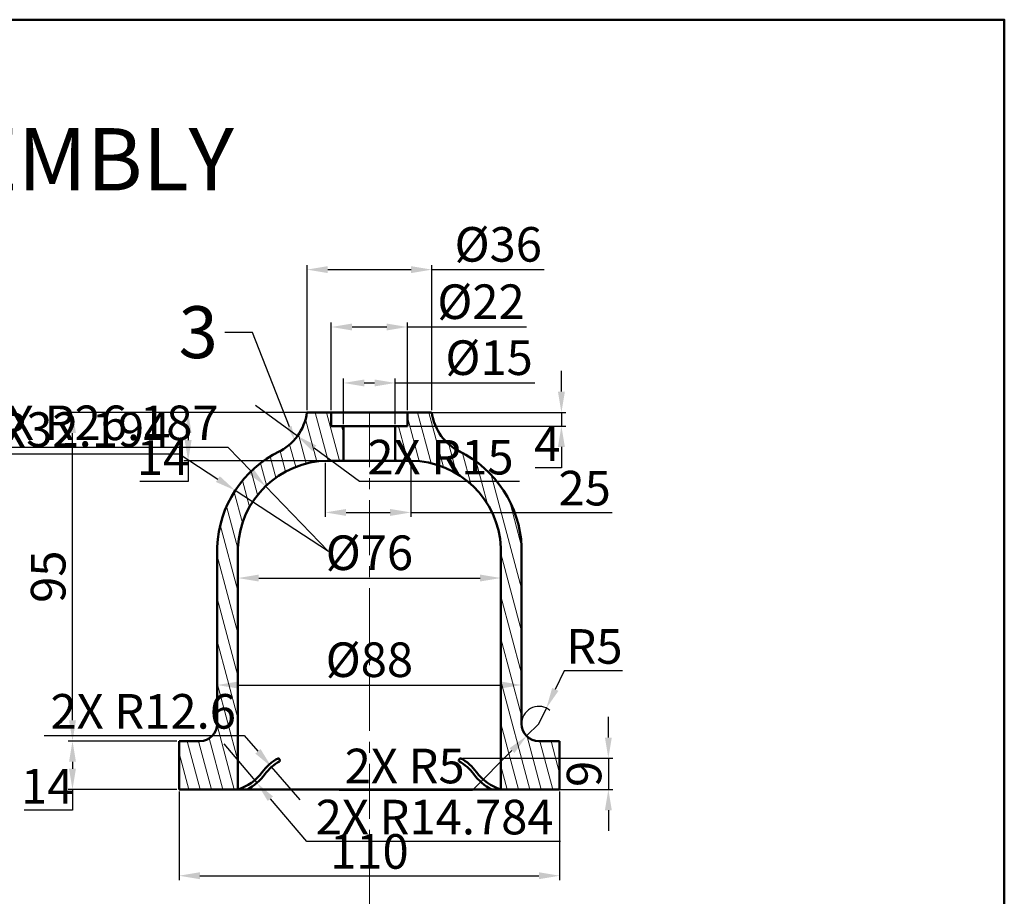
# Model space of a CAD drawing. Units: millimetres. Extents: x 147 to 984, y -369 to 435.
# Tile 10 of 10: x 699 to 984, y 182 to 435. Entities that reach past the tile are written whole.
import ezdxf
from ezdxf import colors
from ezdxf.entities.mleader import LeaderData, LeaderLine
from ezdxf.math import Vec2, Vec3

# ---------------------------------------------------------------- set-up
doc = ezdxf.new("R2010")
doc.units = ezdxf.units.MM
doc.header["$LTSCALE"] = 0.5
doc.linetypes.add('CENTER', pattern=[50.8, 31.75, -6.35, 6.35, -6.35])
for name, color, linetype, lineweight in [('M-CNTR', 1, 'CENTER', 18), ('M-DIMS', 2, 'Continuous', 25), ('M-HATC', 8, 'Continuous', 18), ('M-OUTL', 7, 'Continuous', 50), ('M-TEXT', 7, 'Continuous', 25)]:
    doc.layers.add(name, color=color, linetype=linetype, lineweight=lineweight)
doc.styles.get("Standard").update_dxf_attribs({"font": 'arial.ttf'})
doc.dimstyles.new('ISO-25', dxfattribs={"dimtxt": 10, "dimasz": 6, "dimexe": 1.25, "dimexo": 0.625, "dimtad": 1, "dimtoh": 1, "dimdec": 0, "dimtxsty": 'Standard', "dimcen": 2.5, "dimadec": 0, "dimazin": 0, "dimtfac": 1, "dimtdec": 0, "dimtmove": 0, "dimatfit": 3, "dimfxl": 1, "dimarcsym": 0})

# ---------------------------------------------------------------- blocks, each defined once
blk = doc.blocks.new('*D45')
at = {"layer": 'Defpoints', "color": 0, "transparency": 16777216}
for p in [(745.56, 212.8), (855.56, 212.8), (855.56, 187.86)]:
    blk.add_point(p, dxfattribs=at)
at = {"layer": 'M-DIMS', "color": 0, "lineweight": -2, "transparency": 16777216}
for p, q in [((745.56, 212.17), (745.56, 186.61)), ((855.56, 212.17), (855.56, 186.61)), ((751.56, 187.86), (849.56, 187.86))]:
    blk.add_line(p, q, dxfattribs=at)
at = {"layer": 'M-DIMS', "color": 0, "transparency": 16777216}
for points in [[(751.56, 188.86), (751.56, 186.86), (745.56, 187.86)], [(849.56, 188.86), (849.56, 186.86), (855.56, 187.86)]]:
    blk.add_solid(points, dxfattribs=at)
at = {"layer": 'M-DIMS', "color": 0, "transparency": 16777216, "insert": (800.56, 193.59), "char_height": 10, "attachment_point": 5}
blk.add_mtext('110', dxfattribs=at)
blk = doc.blocks.new('*D46')
at = {"layer": 'Defpoints', "color": 0, "transparency": 16777216}
for p in [(818.59, 363.06), (782.53, 321.8), (818.59, 321.8)]:
    blk.add_point(p, dxfattribs=at)
at = {"layer": 'M-DIMS', "color": 0, "lineweight": -2, "transparency": 16777216}
for p, q in [((782.53, 322.42), (782.53, 364.31)), ((818.59, 322.42), (818.59, 364.31)), ((788.53, 363.06), (812.59, 363.06)), ((818.59, 363.06), (851.04, 363.06))]:
    blk.add_line(p, q, dxfattribs=at)
at = {"layer": 'M-DIMS', "color": 0, "transparency": 16777216}
for points in [[(788.53, 364.06), (788.53, 362.06), (782.53, 363.06)], [(812.59, 364.06), (812.59, 362.06), (818.59, 363.06)]]:
    blk.add_solid(points, dxfattribs=at)
at = {"layer": 'M-DIMS', "color": 0, "transparency": 16777216, "insert": (837.81, 369.07), "char_height": 10, "attachment_point": 5}
blk.add_mtext('%%C36', dxfattribs=at)
blk = doc.blocks.new('*D47')
at = {"layer": 'Defpoints', "color": 0, "transparency": 16777216}
for p in [(811.56, 346.48), (789.56, 321.8), (811.56, 321.8)]:
    blk.add_point(p, dxfattribs=at)
at = {"layer": 'M-DIMS', "color": 0, "lineweight": -2, "transparency": 16777216}
for p, q in [((789.56, 322.42), (789.56, 347.73)), ((811.56, 322.42), (811.56, 347.73)), ((795.56, 346.48), (805.56, 346.48)), ((811.56, 346.48), (846, 346.48))]:
    blk.add_line(p, q, dxfattribs=at)
at = {"layer": 'M-DIMS', "color": 0, "transparency": 16777216}
for points in [[(795.56, 347.48), (795.56, 345.48), (789.56, 346.48)], [(805.56, 347.48), (805.56, 345.48), (811.56, 346.48)]]:
    blk.add_solid(points, dxfattribs=at)
at = {"layer": 'M-DIMS', "color": 0, "transparency": 16777216, "insert": (832.82, 352.49), "char_height": 10, "attachment_point": 5}
blk.add_mtext('%%C22', dxfattribs=at)
blk = doc.blocks.new('*D48')
at = {"layer": 'Defpoints', "color": 0, "transparency": 16777216}
for p in [(808.06, 330.3), (793.06, 317.8), (808.06, 317.8)]:
    blk.add_point(p, dxfattribs=at)
at = {"layer": 'M-DIMS', "color": 0, "lineweight": -2, "transparency": 16777216}
for p, q in [((793.06, 318.42), (793.06, 331.55)), ((799.06, 330.3), (802.06, 330.3)), ((808.06, 318.42), (808.06, 331.55)), ((808.06, 330.3), (848.42, 330.3))]:
    blk.add_line(p, q, dxfattribs=at)
at = {"layer": 'M-DIMS', "color": 0, "transparency": 16777216}
for points in [[(799.06, 331.3), (799.06, 329.3), (793.06, 330.3)], [(802.06, 331.3), (802.06, 329.3), (808.06, 330.3)]]:
    blk.add_solid(points, dxfattribs=at)
at = {"layer": 'M-DIMS', "color": 0, "transparency": 16777216, "insert": (835.16, 336.31), "char_height": 10, "attachment_point": 5}
blk.add_mtext('%%C15', dxfattribs=at)
blk = doc.blocks.new('*D49')
at = {"layer": 'Defpoints', "color": 0, "transparency": 16777216}
for p in [(789.56, 321.8), (748.17, 307.8), (789.56, 307.8)]:
    blk.add_point(p, dxfattribs=at)
at = {"layer": 'M-DIMS', "color": 0, "lineweight": -2, "transparency": 16777216}
for p, q in [((788.93, 321.8), (746.92, 321.8)), ((748.17, 315.8), (748.17, 313.8)), ((788.93, 307.8), (746.92, 307.8)), ((748.17, 307.8), (748.17, 301.8)), ((748.17, 301.8), (734.21, 301.8))]:
    blk.add_line(p, q, dxfattribs=at)
at = {"layer": 'M-DIMS', "color": 0, "transparency": 16777216}
for points in [[(747.17, 315.8), (749.17, 315.8), (748.17, 321.8)], [(747.17, 313.8), (749.17, 313.8), (748.17, 307.8)]]:
    blk.add_solid(points, dxfattribs=at)
at = {"layer": 'M-DIMS', "color": 0, "transparency": 16777216, "insert": (740.88, 307.44), "char_height": 10, "attachment_point": 5}
blk.add_mtext('14', dxfattribs=at)
blk = doc.blocks.new('*D50')
at = {"layer": 'Defpoints', "color": 0, "transparency": 16777216}
for p in [(811.56, 321.8), (811.56, 317.8), (856.07, 317.8)]:
    blk.add_point(p, dxfattribs=at)
at = {"layer": 'M-DIMS', "color": 0, "lineweight": -2, "transparency": 16777216}
for p, q in [((856.07, 327.8), (856.07, 333.8)), ((812.18, 321.8), (857.32, 321.8)), ((856.07, 321.8), (856.07, 317.8)), ((812.18, 317.8), (857.32, 317.8)), ((856.07, 311.8), (856.07, 305.8)), ((856.07, 305.8), (848.52, 305.8))]:
    blk.add_line(p, q, dxfattribs=at)
at = {"layer": 'M-DIMS', "color": 0, "transparency": 16777216}
for points in [[(855.07, 327.8), (857.07, 327.8), (856.07, 321.8)], [(855.07, 311.8), (857.07, 311.8), (856.07, 317.8)]]:
    blk.add_solid(points, dxfattribs=at)
at = {"layer": 'M-DIMS', "color": 0, "transparency": 16777216, "insert": (851.98, 311.42), "char_height": 10, "attachment_point": 5}
blk.add_mtext('4', dxfattribs=at)
blk = doc.blocks.new('*D51')
at = {"layer": 'Defpoints', "color": 0, "transparency": 16777216}
for p in [(756.56, 257.38), (844.56, 257.38), (844.56, 242.99)]:
    blk.add_point(p, dxfattribs=at)
at = {"layer": 'M-DIMS', "color": 0, "lineweight": -2, "transparency": 16777216}
for p, q in [((756.56, 256.75), (756.56, 241.74)), ((844.56, 256.75), (844.56, 241.74)), ((762.56, 242.99), (838.56, 242.99))]:
    blk.add_line(p, q, dxfattribs=at)
at = {"layer": 'M-DIMS', "color": 0, "transparency": 16777216}
for points in [[(762.56, 243.99), (762.56, 241.99), (756.56, 242.99)], [(838.56, 243.99), (838.56, 241.99), (844.56, 242.99)]]:
    blk.add_solid(points, dxfattribs=at)
at = {"layer": 'M-DIMS', "color": 0, "transparency": 16777216, "insert": (800.56, 249), "char_height": 10, "attachment_point": 5}
blk.add_mtext('%%C88', dxfattribs=at)
blk = doc.blocks.new('*D52')
at = {"layer": 'Defpoints', "color": 0, "transparency": 16777216}
for p in [(762.56, 273.91), (838.56, 273.91), (838.56, 273.91)]:
    blk.add_point(p, dxfattribs=at)
at = {"layer": 'M-DIMS', "color": 0, "lineweight": -2, "transparency": 16777216}
for p, q in [((762.56, 274.53), (762.56, 275.16)), ((768.56, 273.91), (832.56, 273.91)), ((838.56, 274.53), (838.56, 275.16))]:
    blk.add_line(p, q, dxfattribs=at)
at = {"layer": 'M-DIMS', "color": 0, "transparency": 16777216}
for points in [[(768.56, 274.91), (768.56, 272.91), (762.56, 273.91)], [(832.56, 274.91), (832.56, 272.91), (838.56, 273.91)]]:
    blk.add_solid(points, dxfattribs=at)
at = {"layer": 'M-DIMS', "color": 0, "transparency": 16777216, "insert": (800.56, 279.92), "char_height": 10, "attachment_point": 5}
blk.add_mtext('%%C76', dxfattribs=at)
blk = doc.blocks.new('*D53')
at = {"layer": 'Defpoints', "color": 0, "transparency": 16777216}
for p in [(745.56, 226.8), (714.74, 212.8), (745.56, 212.8)]:
    blk.add_point(p, dxfattribs=at)
at = {"layer": 'M-DIMS', "color": 0, "lineweight": -2, "transparency": 16777216}
for p, q in [((744.93, 226.8), (713.49, 226.8)), ((714.74, 220.8), (714.74, 218.8)), ((744.93, 212.8), (713.49, 212.8)), ((714.74, 212.8), (714.74, 206.8)), ((714.74, 206.8), (700.77, 206.8))]:
    blk.add_line(p, q, dxfattribs=at)
at = {"layer": 'M-DIMS', "color": 0, "transparency": 16777216}
for points in [[(713.74, 220.8), (715.74, 220.8), (714.74, 226.8)], [(713.74, 218.8), (715.74, 218.8), (714.74, 212.8)]]:
    blk.add_solid(points, dxfattribs=at)
at = {"layer": 'M-DIMS', "color": 0, "transparency": 16777216, "insert": (707.44, 212.44), "char_height": 10, "attachment_point": 5}
blk.add_mtext('14', dxfattribs=at)
blk = doc.blocks.new('*D54')
at = {"layer": 'Defpoints', "color": 0, "transparency": 16777216}
for p in [(714.74, 321.8), (800.56, 321.8), (729.21, 226.8)]:
    blk.add_point(p, dxfattribs=at)
at = {"layer": 'M-DIMS', "color": 0, "lineweight": -2, "transparency": 16777216}
for p, q in [((799.93, 321.8), (713.49, 321.8)), ((714.74, 232.8), (714.74, 315.8)), ((728.58, 226.8), (713.49, 226.8))]:
    blk.add_line(p, q, dxfattribs=at)
at = {"layer": 'M-DIMS', "color": 0, "transparency": 16777216}
for points in [[(713.74, 315.8), (715.74, 315.8), (714.74, 321.8)], [(713.74, 232.8), (715.74, 232.8), (714.74, 226.8)]]:
    blk.add_solid(points, dxfattribs=at)
at = {"layer": 'M-DIMS', "color": 0, "transparency": 16777216, "insert": (709.01, 274.3), "char_height": 10, "attachment_point": 5, "rotation": 90}
blk.add_mtext('95', dxfattribs=at)
blk = doc.blocks.new('*D55')
at = {"layer": 'Defpoints', "color": 0, "transparency": 16777216}
for p in [(826.88, 221.81), (826.88, 212.8), (869.64, 212.8)]:
    blk.add_point(p, dxfattribs=at)
at = {"layer": 'M-DIMS', "color": 0, "lineweight": -2, "transparency": 16777216}
for p, q in [((869.64, 227.81), (869.64, 233.81)), ((827.51, 221.81), (870.89, 221.81)), ((869.64, 221.81), (869.64, 212.8)), ((827.51, 212.8), (870.89, 212.8)), ((869.64, 206.8), (869.64, 200.8))]:
    blk.add_line(p, q, dxfattribs=at)
at = {"layer": 'M-DIMS', "color": 0, "transparency": 16777216}
for points in [[(868.64, 227.81), (870.64, 227.81), (869.64, 221.81)], [(868.64, 206.8), (870.64, 206.8), (869.64, 212.8)]]:
    blk.add_solid(points, dxfattribs=at)
at = {"layer": 'M-DIMS', "color": 0, "transparency": 16777216, "insert": (863.91, 217.3), "char_height": 10, "attachment_point": 5, "rotation": 90}
blk.add_mtext('9', dxfattribs=at)
blk = doc.blocks.new('*D56')
at = {"layer": 'Defpoints', "color": 0, "transparency": 16777216}
for p in [(851.72, 236.31), (849.56, 231.8)]:
    blk.add_point(p, dxfattribs=at)
at = {"layer": 'M-DIMS', "color": 0, "lineweight": -2, "transparency": 16777216}
for p, q in [((856.89, 247.13), (854.3, 241.72)), ((873.72, 247.13), (856.89, 247.13)), ((849.56, 231.8), (851.72, 236.31))]:
    blk.add_line(p, q, dxfattribs=at)
blk.add_arc((849.56, 231.8), 5, 50.1085, 172.838, dxfattribs=at)
at = {"layer": 'M-DIMS', "color": 0, "transparency": 16777216}
blk.add_solid([(853.4, 242.15), (855.21, 241.29), (851.72, 236.31)], dxfattribs=at)
at = {"layer": 'M-DIMS', "color": 0, "transparency": 16777216, "insert": (865.62, 252.84), "char_height": 10, "attachment_point": 5}
blk.add_mtext('R5', dxfattribs=at)
blk = doc.blocks.new('*D57')
at = {"layer": 'Defpoints', "color": 0, "transparency": 16777216}
for p in [(787.82, 307.8), (812.56, 307.8), (812.56, 292.87)]:
    blk.add_point(p, dxfattribs=at)
at = {"layer": 'M-DIMS', "color": 0, "lineweight": -2, "transparency": 16777216}
for p, q in [((787.82, 307.17), (787.82, 291.62)), ((812.56, 307.17), (812.56, 291.62)), ((793.82, 292.87), (806.56, 292.87)), ((812.56, 292.87), (870.69, 292.87))]:
    blk.add_line(p, q, dxfattribs=at)
at = {"layer": 'M-DIMS', "color": 0, "transparency": 16777216}
for points in [[(793.82, 293.87), (793.82, 291.87), (787.82, 292.87)], [(806.56, 293.87), (806.56, 291.87), (812.56, 292.87)]]:
    blk.add_solid(points, dxfattribs=at)
at = {"layer": 'M-DIMS', "color": 0, "transparency": 16777216, "insert": (862.78, 298.6), "char_height": 10, "attachment_point": 5}
blk.add_mtext('25', dxfattribs=at)
blk = doc.blocks.new('*U62')
at = {"layer": 'M-CNTR', "color": 0, "transparency": 16777216}
blk.add_line((0, 99.41), (0, -106.28), dxfattribs=at)
blk = doc.blocks.new('*D168')
at = {"layer": 'Defpoints', "color": 0, "ltscale": 0.5, "transparency": 16777216}
for p in [(761.78, 299.23), (788.72, 281.61)]:
    blk.add_point(p, dxfattribs=at)
at = {"layer": 'M-DIMS', "color": 0, "lineweight": -2, "ltscale": 0.5, "transparency": 16777216}
for p, q in [((672.29, 309.8), (745.62, 309.8)), ((745.62, 309.8), (756.76, 302.52)), ((788.72, 281.61), (761.78, 299.23))]:
    blk.add_line(p, q, dxfattribs=at)
at = {"layer": 'M-DIMS', "color": 0, "ltscale": 0.5, "transparency": 16777216}
blk.add_solid([(757.31, 303.35), (756.21, 301.68), (761.78, 299.23)], dxfattribs=at)
at = {"layer": 'M-DIMS', "color": 0, "ltscale": 0.5, "transparency": 16777216, "insert": (708.64, 315.54), "char_height": 10, "attachment_point": 5}
blk.add_mtext('2X R32.194', dxfattribs=at)
blk = doc.blocks.new('*D169')
at = {"layer": 'Defpoints', "color": 0, "ltscale": 0.5, "transparency": 16777216}
for p in [(770.53, 300.44), (788.72, 281.61)]:
    blk.add_point(p, dxfattribs=at)
at = {"layer": 'M-DIMS', "color": 0, "lineweight": -2, "ltscale": 0.5, "transparency": 16777216}
for p, q in [((686.24, 311.74), (759.61, 311.74)), ((759.61, 311.74), (766.36, 304.76)), ((788.72, 281.61), (770.53, 300.44))]:
    blk.add_line(p, q, dxfattribs=at)
at = {"layer": 'M-DIMS', "color": 0, "ltscale": 0.5, "transparency": 16777216}
blk.add_solid([(767.08, 305.45), (765.64, 304.06), (770.53, 300.44)], dxfattribs=at)
at = {"layer": 'M-DIMS', "color": 0, "ltscale": 0.5, "transparency": 16777216, "insert": (722.61, 317.47), "char_height": 10, "attachment_point": 5}
blk.add_mtext('2X R26.187', dxfattribs=at)
blk = doc.blocks.new('*D170')
at = {"layer": 'Defpoints', "color": 0, "ltscale": 0.5, "transparency": 16777216}
for p in [(767.67, 323.84), (779.76, 314.97)]:
    blk.add_point(p, dxfattribs=at)
at = {"layer": 'M-DIMS', "color": 0, "lineweight": -2, "ltscale": 0.5, "transparency": 16777216}
for p, q in [((767.67, 323.84), (779.76, 314.97)), ((797.67, 301.83), (784.6, 311.42)), ((843.93, 301.83), (797.67, 301.83))]:
    blk.add_line(p, q, dxfattribs=at)
at = {"layer": 'M-DIMS', "color": 0, "ltscale": 0.5, "transparency": 16777216}
blk.add_solid([(785.19, 312.23), (784.01, 310.61), (779.76, 314.97)], dxfattribs=at)
at = {"layer": 'M-DIMS', "color": 0, "ltscale": 0.5, "transparency": 16777216, "insert": (821.11, 307.56), "char_height": 10, "attachment_point": 5}
blk.add_mtext('2X R15', dxfattribs=at)
blk = doc.blocks.new('*D171')
at = {"layer": 'Defpoints', "color": 0, "ltscale": 0.5, "transparency": 16777216}
for p in [(758.45, 225.95), (768.03, 214.7)]:
    blk.add_point(p, dxfattribs=at)
at = {"layer": 'M-DIMS', "color": 0, "lineweight": -2, "ltscale": 0.5, "transparency": 16777216}
for p, q in [((758.45, 225.95), (768.03, 214.7)), ((782.44, 197.79), (771.93, 210.13)), ((855.77, 197.79), (782.44, 197.79))]:
    blk.add_line(p, q, dxfattribs=at)
at = {"layer": 'M-DIMS', "color": 0, "ltscale": 0.5, "transparency": 16777216}
blk.add_solid([(772.69, 210.78), (771.16, 209.48), (768.03, 214.7)], dxfattribs=at)
at = {"layer": 'M-DIMS', "color": 0, "ltscale": 0.5, "transparency": 16777216, "insert": (819.42, 203.52), "char_height": 10, "attachment_point": 5}
blk.add_mtext('2X R14.784', dxfattribs=at)
blk = doc.blocks.new('*D172')
at = {"layer": 'Defpoints', "color": 0, "ltscale": 0.5, "transparency": 16777216}
for p in [(772.28, 219.3), (780.56, 209.8)]:
    blk.add_point(p, dxfattribs=at)
at = {"layer": 'M-DIMS', "color": 0, "lineweight": -2, "ltscale": 0.5, "transparency": 16777216}
for p, q in [((706.59, 228.35), (764.41, 228.35)), ((764.41, 228.35), (768.35, 223.83)), ((780.56, 209.8), (772.28, 219.3))]:
    blk.add_line(p, q, dxfattribs=at)
at = {"layer": 'M-DIMS', "color": 0, "ltscale": 0.5, "transparency": 16777216}
blk.add_solid([(769.1, 224.48), (767.59, 223.17), (772.28, 219.3)], dxfattribs=at)
at = {"layer": 'M-DIMS', "color": 0, "ltscale": 0.5, "transparency": 16777216, "insert": (735.18, 234.08), "char_height": 10, "attachment_point": 5}
blk.add_mtext('2X R12.6', dxfattribs=at)
blk = doc.blocks.new('*D173')
at = {"layer": 'Defpoints', "color": 0, "ltscale": 0.5, "transparency": 16777216}
for p in [(849.56, 231.8), (846.02, 228.26)]:
    blk.add_point(p, dxfattribs=at)
at = {"layer": 'M-DIMS', "color": 0, "lineweight": -2, "ltscale": 0.5, "transparency": 16777216}
for p, q in [((849.56, 231.8), (846.02, 228.26)), ((830.32, 212.55), (841.78, 224.02)), ((791.83, 212.55), (830.32, 212.55))]:
    blk.add_line(p, q, dxfattribs=at)
at = {"layer": 'M-DIMS', "color": 0, "ltscale": 0.5, "transparency": 16777216}
blk.add_solid([(841.07, 224.72), (842.49, 223.31), (846.02, 228.26)], dxfattribs=at)
at = {"layer": 'M-DIMS', "color": 0, "ltscale": 0.5, "transparency": 16777216, "insert": (810.76, 218.28), "char_height": 10, "attachment_point": 5}
blk.add_mtext('2X R5', dxfattribs=at)

msp = doc.modelspace()

# ---------------------------------------------------------------- hatches: boundary and pattern name
at = {"layer": 'M-HATC'}
h = msp.add_hatch(dxfattribs=at)
h.set_pattern_fill('ANSI31', color=256, angle=60)
h.set_pattern_definition([(105, (-285.9122, 3e-14), (-3.0668145, -0.8217505), [])])
h.paths.add_polyline_path([(751.5575, 226.7953), (745.5575, 226.7953), (745.5575, 212.7953), (762.5575, 212.7953), (762.5575, 282.6726, -0.40053029), (788.5575, 307.7953), (793.0575, 307.7953), (793.0575, 317.7953), (789.5575, 317.7953), (789.5575, 321.7953), (782.5259, 321.7953, -0.25326572), (774.0809, 310.2801, 0.27051223), (756.5575, 282.9569), (756.5575, 231.7953, -0.41421356)])
h.paths.add_polyline_path([(838.5575, 212.7953), (855.5575, 212.7953), (855.5575, 226.7953), (849.5575, 226.7953, -0.41421356), (844.5575, 231.7953), (844.5575, 282.9569, 0.27051223), (827.0341, 310.2801, -0.25326572), (818.5891, 321.7953), (811.5575, 321.7953), (811.5575, 317.7953), (808.0575, 317.7953), (808.0575, 307.7953), (812.2269, 307.7953, -0.40419762), (838.5575, 282.6726)])

# ---------------------------------------------------------------- linework, layer by layer
at = {"layer": 'M-CNTR'}
msp.add_line((800.5575, 321.7953), (800.5575, 4.2226), dxfattribs=at)
at = {"layer": 'M-OUTL'}
for p, q in [((800.5575, 321.7953), (782.5259, 321.7953)), ((789.5575, 321.7953), (789.5575, 317.7953)), ((811.5575, 321.7953), (789.5575, 321.7953)), ((800.5575, 321.7953), (818.5575, 321.7953)), ((811.5575, 317.7953), (811.5575, 321.7953)), ((789.5575, 317.7953), (811.5575, 317.7953)), ((793.0575, 307.7953), (793.0575, 317.7953)), ((808.0575, 307.7953), (808.0575, 317.7953)), ((788.5575, 307.7953), (812.5575, 307.7953)), ((800.5575, 307.7953), (793.0575, 307.7953)), ((800.5575, 307.7953), (808.0575, 307.7953)), ((756.5575, 282.9569), (756.5575, 231.7953)), ((762.5575, 282.6726), (762.5575, 212.7953)), ((838.5575, 282.6726), (838.5575, 212.7953)), ((844.5575, 282.9569), (844.5575, 231.7953)), ((751.5575, 226.7953), (745.5575, 226.7953)), ((745.5575, 226.7953), (745.5575, 212.7953)), ((855.5575, 226.7953), (849.5575, 226.7953)), ((855.5575, 212.7953), (855.5575, 226.7953)), ((745.5575, 212.7953), (855.5575, 212.7953))]:
    msp.add_line(p, q, dxfattribs=at)
at = {"layer": 'M-OUTL', "ltscale": 0.5}
msp.add_lwpolyline([(147.3511, 435.3078), (984.0884, 435.3078), (984.0884, -369.4968), (147.3511, -369.4968)], close=True, dxfattribs=at)
at = {"layer": 'M-OUTL'}
for points in [[(774.1541, 221.7953, 0.11345998), (769.5575, 217.7953, -0.16001287), (762.5575, 212.7953)], [(774.6249, 220.9131, 0.11350329), (770.365, 217.2055, -0.11654733), (765.1892, 212.7953, -0.11654733)], [(826.4901, 220.9131, -0.11350329), (830.75, 217.2055, 0.11654733), (835.9258, 212.7953, 0.11654733)], [(826.9608, 221.7953, -0.11345998), (831.5575, 217.7953, 0.16001287), (838.5575, 212.7953)]]:
    msp.add_lwpolyline(points, format="xyb", dxfattribs=at)
for centre, radius, start, end in [((767.6657, 323.8391), 15, 295.320066, 352.168918), ((833.4492, 323.8391), 15, 187.831082, 244.679934), ((788.7228, 281.6089), 32.1935, 115.951335, 177.672078), ((812.3922, 281.6089), 32.1935, 2.327922, 64.048665), ((788.7228, 281.6089), 26.1869, 90.361688, 177.672078), ((812.3922, 281.6089), 26.1869, 2.327922, 89.638312), ((751.5575, 231.7953), 5, 270, 0), ((849.5575, 231.7953), 5, 180, 270)]:
    msp.add_arc(centre, radius, start, end, dxfattribs=at)
for points in [[(774.1541, 221.7953), (774.4482, 221.9523), (774.919, 221.07), (774.6249, 220.9131)], [(826.9608, 221.7953), (826.6668, 221.9523), (826.196, 221.07), (826.4901, 220.9131)]]:
    msp.add_open_spline(points, degree=3, dxfattribs=at)

# ---------------------------------------------------------------- block references
at = {"layer": 'M-CNTR'}
msp.add_blockref('*U62', (800.5575, 94.5279), dxfattribs=at)

# ---------------------------------------------------------------- texts
at = {"layer": 'M-TEXT', "ltscale": 0.5, "insert": (313.9939, 403.9552), "char_height": 18, "attachment_point": 1}
msp.add_mtext_dynamic_manual_height_columns('\\pxqc;RUBBER-SEATED VALVE ASSEMBLY', width=497.441574, gutter_width=12.5, heights=[0], dxfattribs=at)

# ---------------------------------------------------------------- dimensions: what is measured, and where the dimension line sits
at = {"layer": 'M-DIMS'}
for base, p1, p2, picture, middle in [((818.5891, 363.064), (782.5259, 321.7953), (818.5891, 321.7953), '*D46', (837.813, 363.064)), ((811.5575, 346.4776), (789.5575, 321.7953), (811.5575, 321.7953), '*D47', (832.8203, 346.4776)), ((808.0575, 330.2961), (793.0575, 317.7953), (808.0575, 317.7953), '*D48', (835.1559, 330.2961))]:
    dim = msp.add_linear_dim(base=base, p1=p1, p2=p2, text='%%C<>', dimstyle='ISO-25', override={"dimclrd": 0, "dimclre": 0, "dimclrt": 0}, dxfattribs=at)
    dim.commit()
    dim.dimension.update_dxf_attribs({"geometry": picture, "text_midpoint": middle, "dimtype": 160})
for base, p1, p2, picture, middle in [((856.065, 317.7953), (811.5575, 321.7953), (811.5575, 317.7953), '*D50', (851.9816, 311.4203)), ((714.736, 321.7953), (729.2093, 226.7953), (800.5575, 321.7953), '*D54', (709.0053, 274.2953)), ((748.1725, 307.7953), (789.5575, 321.7953), (789.5575, 307.7953), '*D49', (740.8763, 307.4408)), ((869.638, 212.7953), (826.8815, 221.8139), (826.8815, 212.7953), '*D55', (863.9073, 217.3046)), ((714.736, 212.7953), (745.5575, 226.7953), (745.5575, 212.7953), '*D53', (707.4398, 212.4408))]:
    dim = msp.add_linear_dim(base=base, p1=p1, p2=p2, angle=90, dimstyle='ISO-25', override={"dimclrd": 0, "dimclre": 0, "dimclrt": 0}, dxfattribs=at)
    dim.commit()
    dim.dimension.update_dxf_attribs({"geometry": picture, "text_midpoint": middle})
at = {"layer": 'M-DIMS', "ltscale": 0.5}
for mpoint, picture, middle in [((761.7807, 299.2312), '*D168', (708.6398, 309.8046)), ((770.5262, 300.4408), '*D169', (722.6122, 311.7399))]:
    dim = msp.add_radius_dim(center=(788.7228, 281.6089), mpoint=mpoint, text='2X <>', dimstyle='ISO-25', override={"dimdec": 3, "dimlfac": 1, "dimrnd": 0, "dimzin": 0, "dimdsep": 46, "dimlunit": 2}, dxfattribs=at)
    dim.commit()
    dim.dimension.update_dxf_attribs({"geometry": picture, "text_midpoint": middle, "dimtype": 164})
for center, mpoint, override, picture, middle in [((767.6657, 323.8391), (779.7616, 314.9683), {"dimdec": 0, "dimlfac": 1, "dimrnd": 0, "dimzin": 0, "dimdsep": 46, "dimlunit": 2}, '*D170', (821.1114, 307.5635)), ((780.556, 209.7974), (772.2848, 219.3013), {"dimdec": 1, "dimlfac": 1, "dimrnd": 0, "dimzin": 0, "dimdsep": 46, "dimlunit": 2}, '*D172', (735.1836, 234.0839)), ((849.5575, 231.7953), (846.022, 228.2598), {"dimdec": 0, "dimlfac": 1, "dimrnd": 0, "dimzin": 0, "dimdsep": 46, "dimlunit": 2}, '*D173', (810.762, 218.2847)), ((758.4456, 225.9519), (768.0341, 214.6988), {"dimdec": 3, "dimlfac": 1, "dimrnd": 0, "dimzin": 0, "dimdsep": 46, "dimlunit": 2}, '*D171', (819.4153, 203.5231))]:
    dim = msp.add_radius_dim(center=center, mpoint=mpoint, text='2X <>', dimstyle='ISO-25', override=override, dxfattribs=at)
    dim.commit()
    dim.dimension.update_dxf_attribs({"geometry": picture, "text_midpoint": middle})
at = {"layer": 'M-DIMS'}
dim = msp.add_linear_dim(base=(812.5575, 292.8668), p1=(787.8168, 307.7953), p2=(812.5575, 307.7953), dimstyle='ISO-25', override={"dimclrd": 0, "dimclre": 0, "dimclrt": 0}, dxfattribs=at)
dim.commit()
dim.dimension.update_dxf_attribs({"geometry": '*D57', "text_midpoint": (862.782, 292.8668), "dimtype": 160})
for base, p1, p2, picture, middle in [((838.5575, 273.9067), (762.5575, 273.9067), (838.5575, 273.9067), '*D52', (800.5575, 279.9171)), ((844.5575, 242.9853), (756.5575, 257.3761), (844.5575, 257.3761), '*D51', (800.5575, 248.9957))]:
    dim = msp.add_linear_dim(base=base, p1=p1, p2=p2, text='%%C<>', dimstyle='ISO-25', override={"dimclrd": 0, "dimclre": 0, "dimclrt": 0}, dxfattribs=at)
    dim.commit()
    dim.dimension.update_dxf_attribs({"geometry": picture, "text_midpoint": middle})
dim = msp.add_radius_dim(center=(849.5575, 231.7953), mpoint=(851.7154, 236.3057), dimstyle='ISO-25', override={"dimclrd": 0, "dimclre": 0, "dimclrt": 0}, dxfattribs=at)
dim.commit()
dim.dimension.update_dxf_attribs({"geometry": '*D56', "text_midpoint": (865.6195, 252.8409)})
dim = msp.add_linear_dim(base=(855.5575, 187.8566), p1=(745.5575, 212.7953), p2=(855.5575, 212.7953), dimstyle='ISO-25', override={"dimclrd": 0, "dimclre": 0, "dimclrt": 0}, dxfattribs=at)
dim.commit()
dim.dimension.update_dxf_attribs({"geometry": '*D45', "text_midpoint": (800.5575, 193.5873)})

# ---------------------------------------------------------------- leaders
at = {"layer": 'M-TEXT'}
ml = msp.add_multileader_mtext('Standard', dxfattribs=at)
ml.set_content('3', color=256)
ml.set_leader_properties()
ml.build(insert=Vec2(0, 0))
ctx = ml.context
ctx.base_point, ctx.char_height, ctx.plane_origin = Vec3(744.9427, 344.8456), 15, Vec3(778.9148, 313.9165)
ctx.text_align_type = 2
notes = []
notes.append((ctx, [(0, (1, 1, 0), (766.7653, 344.8456), (-1, 0), 8, [(0, [(778.9148, 313.9165)], 0, [])])]))
ctx.mtext.insert, ctx.mtext.alignment, ctx.mtext.flow_direction = Vec3(756.7653, 352.4786), 3, 5
for ctx, leaders in notes:
    for number, flags, end, landing, length, lines in leaders:
        leader = LeaderData()
        leader.index, (leader.has_last_leader_line, leader.has_dogleg_vector, leader.attachment_direction) = number, flags
        leader.last_leader_point, leader.dogleg_vector, leader.dogleg_length = Vec3(end), Vec3(landing), length
        for number, points, colour, breaks in lines:
            line = LeaderLine()
            line.index, line.vertices, line.color, line.breaks = number, Vec3.list(points), colors.encode_raw_color(colour), breaks
            leader.lines.append(line)
        ctx.leaders.append(leader)

doc.saveas('drawing.dxf')
